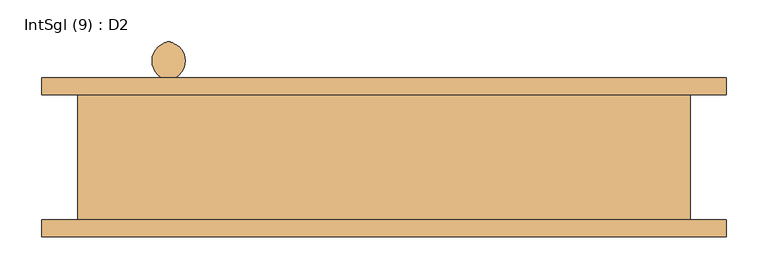
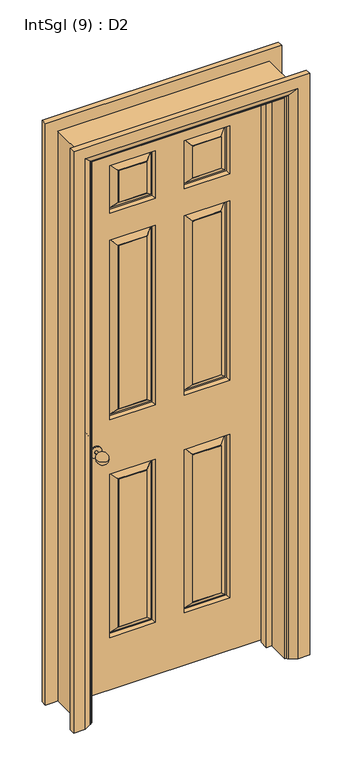
"""IFC4 building model written with IfcOpenShell, lengths in millimetres: door geometry, IntSgl (9) : D2."""

from ifc_helpers import new_model, si_unit, point, frame, origin, place, context, project, spatial, polyline, circle_curve, ellipse_curve, trimmed, outline, extrude, faceted_brep, source, transform, mapped, element, save
from ifc_brep_helpers import plane_surface, cylinder_surface, revolved_surface, advanced_brep


def intsgl_9_d2_8283ee4d(model_context):
    return source(origin(), model_context, "Body", "SolidModel", [
        advanced_brep(
        [(-253.0, 18.0, 900.0), (-258.0, -26.437411, 900.0), (-263.0, 18.0, 900.0), (-263.0, 33.0, 900.0), (-253.0, 33.0, 900.0), (-278.0, 37.0, 900.0), (-238.0, 37.0, 900.0), (-278.0, 33.0, 900.0), (-238.0, 33.0, 900.0)],
        [
            (0, 1, circle_curve(frame((-261.1884862, -3.5786495, 900.0), z_axis=(0.0, 0.0, -1.0), x_axis=(0.0, 1.0, 0.0)), 23.0800654)),
            (1, 2, circle_curve(frame((-254.8115138, -3.5786495, 900.0), z_axis=(0.0, 0.0, -1.0), x_axis=(0.0, 1.0, 0.0)), 23.0800654)),
            (2, 0, circle_curve(frame((-258.0, 18.0, 900.0), z_axis=(0.0, -1.0, 0.0), x_axis=(-1.0, 0.0, 0.0)), 5.0)),
            (0, 2, circle_curve(frame((-258.0, 18.0, 900.0), z_axis=(0.0, -1.0, 0.0), x_axis=(-1.0, 0.0, 0.0)), 5.0)),
            (2, 3),
            (3, 4, circle_curve(frame((-258.0, 33.0, 900.0), z_axis=(0.0, -1.0, 0.0), x_axis=(-1.0, 0.0, 0.0)), 5.0)),
            (4, 0),
            (4, 3, circle_curve(frame((-258.0, 33.0, 900.0), z_axis=(0.0, -1.0, 0.0), x_axis=(-1.0, 0.0, 0.0)), 5.0)),
            (5, 6, circle_curve(frame((-258.0, 37.0, 900.0), z_axis=(0.0, 1.0, 0.0), x_axis=(1.0, 0.0, 0.0)), 20.0)),
            (6, 5, circle_curve(frame((-258.0, 37.0, 900.0), z_axis=(0.0, 1.0, 0.0), x_axis=(1.0, 0.0, 0.0)), 20.0)),
            (7, 8, circle_curve(frame((-258.0, 33.0, 900.0), z_axis=(0.0, -1.0, 0.0), x_axis=(1.0, 0.0, 0.0)), 20.0)),
            (8, 7, circle_curve(frame((-258.0, 33.0, 900.0), z_axis=(0.0, -1.0, 0.0), x_axis=(1.0, 0.0, 0.0)), 20.0)),
            (6, 8),
            (7, 5),
        ],
        [
            revolved_surface(trimmed(ellipse_curve(frame((-254.8115138, -3.5786495, 900.0), z_axis=(0.0, 0.0, -1.0), x_axis=(0.0, 1.0, 0.0)), 23.0800654, 23.0800654), [point((-258.0, -26.437411, 900.0))], [point((-263.0, 18.0, 900.0))], True, "CARTESIAN"), (-258.0, 33.0, 900.0), (0.0, 1.0, 0.0)),
            cylinder_surface(frame((-258.0, 33.0, 900.0), z_axis=(0.0, 1.0, 0.0), x_axis=(-1.0, 0.0, 0.0)), 5.0),
            plane_surface(frame((-238.0, 37.0, 900.0), z_axis=(0.0, 1.0, 0.0), x_axis=(0.0, 0.0, 1.0))),
            plane_surface(frame((-238.0, 33.0, 900.0), z_axis=(0.0, -1.0, 0.0), x_axis=(0.0, 0.0, -1.0))),
            cylinder_surface(frame((-258.0, 33.0, 900.0), z_axis=(0.0, 1.0, 0.0), x_axis=(1.0, 0.0, 0.0)), 20.0),
        ],
        [
            (0, [[1, 2, 3]]),
            (0, [[-1, 4, -2]]),
            (1, [[5, 6, 7, -3]]),
            (1, [[-7, 8, -5, -4]]),
            (2, [[9, 10]]),
            (3, [[11, 12], [-8, -6]]),
            (4, [[13, -11, 14, -10]]),
            (4, [[-14, -12, -13, -9]]),
        ],
    ),
        advanced_brep(
        [(-253.0, 94.0, 900.0), (-263.0, 94.0, 900.0), (-258.0, 138.437411, 900.0), (-253.0, 79.0, 900.0), (-263.0, 79.0, 900.0), (-278.0, 75.0, 900.0), (-238.0, 75.0, 900.0), (-278.0, 79.0, 900.0), (-238.0, 79.0, 900.0)],
        [
            (0, 1, circle_curve(frame((-258.0, 94.0, 900.0), z_axis=(0.0, 1.0, 0.0), x_axis=(-1.0, 0.0, 0.0)), 5.0)),
            (1, 2, circle_curve(frame((-254.8115138, 115.5786495, 900.0), z_axis=(0.0, 0.0, -1.0), x_axis=(0.0, -1.0, 0.0)), 23.0800654)),
            (2, 0, circle_curve(frame((-261.1884862, 115.5786495, 900.0), z_axis=(0.0, 0.0, -1.0), x_axis=(0.0, -1.0, 0.0)), 23.0800654)),
            (1, 0, circle_curve(frame((-258.0, 94.0, 900.0), z_axis=(0.0, 1.0, 0.0), x_axis=(-1.0, 0.0, 0.0)), 5.0)),
            (0, 3),
            (3, 4, circle_curve(frame((-258.0, 79.0, 900.0), z_axis=(0.0, 1.0, 0.0), x_axis=(-1.0, 0.0, 0.0)), 5.0)),
            (4, 1),
            (4, 3, circle_curve(frame((-258.0, 79.0, 900.0), z_axis=(0.0, 1.0, 0.0), x_axis=(-1.0, 0.0, 0.0)), 5.0)),
            (5, 6, circle_curve(frame((-258.0, 75.0, 900.0), z_axis=(0.0, -1.0, 0.0), x_axis=(1.0, 0.0, 0.0)), 20.0)),
            (6, 5, circle_curve(frame((-258.0, 75.0, 900.0), z_axis=(0.0, -1.0, 0.0), x_axis=(1.0, 0.0, 0.0)), 20.0)),
            (7, 8, circle_curve(frame((-258.0, 79.0, 900.0), z_axis=(0.0, 1.0, 0.0), x_axis=(1.0, 0.0, 0.0)), 20.0)),
            (8, 7, circle_curve(frame((-258.0, 79.0, 900.0), z_axis=(0.0, 1.0, 0.0), x_axis=(1.0, 0.0, 0.0)), 20.0)),
            (5, 7),
            (8, 6),
        ],
        [
            revolved_surface(trimmed(ellipse_curve(frame((-254.8115138, 115.5786495, 900.0), z_axis=(0.0, 0.0, 1.0), x_axis=(0.0, -1.0, 0.0)), 23.0800654, 23.0800654), [point((-258.0, 138.437411, 900.0))], [point((-263.0, 94.0, 900.0))], True, "CARTESIAN"), (-258.0, 79.0, 900.0), (0.0, -1.0, 0.0)),
            cylinder_surface(frame((-258.0, 79.0, 900.0), z_axis=(0.0, -1.0, 0.0), x_axis=(-1.0, 0.0, 0.0)), 5.0),
            plane_surface(frame((-238.0, 75.0, 900.0), z_axis=(0.0, -1.0, 0.0), x_axis=(0.0, 0.0, 1.0))),
            plane_surface(frame((-238.0, 79.0, 900.0), z_axis=(0.0, 1.0, 0.0), x_axis=(0.0, 0.0, -1.0))),
            cylinder_surface(frame((-258.0, 79.0, 900.0), z_axis=(0.0, -1.0, 0.0), x_axis=(1.0, 0.0, 0.0)), 20.0),
        ],
        [
            (0, [[1, 2, 3]]),
            (0, [[-2, 4, -3]]),
            (1, [[-1, 5, 6, 7]]),
            (1, [[-4, -7, 8, -5]]),
            (2, [[9, 10]]),
            (3, [[11, 12], [-6, -8]]),
            (4, [[-9, 13, -12, 14]]),
            (4, [[-10, -14, -11, -13]]),
        ],
    ),
        faceted_brep([(-333.0, 37.0, 2058.0), (-333.0, 37.0, 8.0), (333.0, 37.0, 8.0), (333.0, 37.0, 2058.0), (-50.0, 37.0, 800.0), (-50.0, 37.0, 200.0), (-208.0, 37.0, 200.0), (-208.0, 37.0, 800.0), (208.0, 37.0, 800.0), (208.0, 37.0, 200.0), (50.0, 37.0, 200.0), (50.0, 37.0, 800.0), (-50.0, 37.0, 1658.0), (-50.0, 37.0, 1000.0), (-208.0, 37.0, 1000.0), (-208.0, 37.0, 1658.0), (208.0, 37.0, 1658.0), (208.0, 37.0, 1000.0), (50.0, 37.0, 1000.0), (50.0, 37.0, 1658.0), (-50.0, 37.0, 1933.0), (-50.0, 37.0, 1758.0), (-208.0, 37.0, 1758.0), (-208.0, 37.0, 1933.0), (208.0, 37.0, 1933.0), (208.0, 37.0, 1758.0), (50.0, 37.0, 1758.0), (50.0, 37.0, 1933.0), (-80.0, 37.0, 230.0), (-80.0, 37.0, 770.0), (-178.0, 37.0, 770.0), (-178.0, 37.0, 230.0), (178.0, 37.0, 230.0), (178.0, 37.0, 770.0), (80.0, 37.0, 770.0), (80.0, 37.0, 230.0), (-80.0, 37.0, 1030.0), (-80.0, 37.0, 1628.0), (-178.0, 37.0, 1628.0), (-178.0, 37.0, 1030.0), (178.0, 37.0, 1030.0), (178.0, 37.0, 1628.0), (80.0, 37.0, 1628.0), (80.0, 37.0, 1030.0), (-80.0, 37.0, 1788.0), (-80.0, 37.0, 1903.0), (-178.0, 37.0, 1903.0), (-178.0, 37.0, 1788.0), (178.0, 37.0, 1788.0), (178.0, 37.0, 1903.0), (80.0, 37.0, 1903.0), (80.0, 37.0, 1788.0), (-333.0, 75.0, 2058.0), (333.0, 75.0, 2058.0), (333.0, 75.0, 8.0), (-333.0, 75.0, 8.0), (50.0, 75.0, 800.0), (50.0, 75.0, 200.0), (208.0, 75.0, 200.0), (208.0, 75.0, 800.0), (-208.0, 75.0, 800.0), (-208.0, 75.0, 200.0), (-50.0, 75.0, 200.0), (-50.0, 75.0, 800.0), (50.0, 75.0, 1658.0), (50.0, 75.0, 1000.0), (208.0, 75.0, 1000.0), (208.0, 75.0, 1658.0), (-208.0, 75.0, 1658.0), (-208.0, 75.0, 1000.0), (-50.0, 75.0, 1000.0), (-50.0, 75.0, 1658.0), (50.0, 75.0, 1933.0), (50.0, 75.0, 1758.0), (208.0, 75.0, 1758.0), (208.0, 75.0, 1933.0), (-208.0, 75.0, 1933.0), (-208.0, 75.0, 1758.0), (-50.0, 75.0, 1758.0), (-50.0, 75.0, 1933.0), (80.0, 75.0, 230.0), (80.0, 75.0, 770.0), (178.0, 75.0, 770.0), (178.0, 75.0, 230.0), (-178.0, 75.0, 230.0), (-178.0, 75.0, 770.0), (-80.0, 75.0, 770.0), (-80.0, 75.0, 230.0), (80.0, 75.0, 1030.0), (80.0, 75.0, 1628.0), (178.0, 75.0, 1628.0), (178.0, 75.0, 1030.0), (-178.0, 75.0, 1030.0), (-178.0, 75.0, 1628.0), (-80.0, 75.0, 1628.0), (-80.0, 75.0, 1030.0), (80.0, 75.0, 1788.0), (80.0, 75.0, 1903.0), (178.0, 75.0, 1903.0), (178.0, 75.0, 1788.0), (-178.0, 75.0, 1788.0), (-178.0, 75.0, 1903.0), (-80.0, 75.0, 1903.0), (-80.0, 75.0, 1788.0), (80.0, 74.0, 230.0), (80.0, 74.0, 770.0), (58.0, 60.0, 208.0), (58.0, 60.0, 792.0), (78.0, 74.0, 772.0), (78.0, 74.0, 228.0), (53.0, 60.0, 797.0), (53.0, 60.0, 203.0), (178.0, 74.0, 770.0), (200.0, 60.0, 792.0), (180.0, 74.0, 772.0), (205.0, 60.0, 797.0), (178.0, 74.0, 230.0), (200.0, 60.0, 208.0), (180.0, 74.0, 228.0), (205.0, 60.0, 203.0), (-178.0, 74.0, 230.0), (-178.0, 74.0, 770.0), (-200.0, 60.0, 208.0), (-200.0, 60.0, 792.0), (-180.0, 74.0, 772.0), (-180.0, 74.0, 228.0), (-205.0, 60.0, 797.0), (-205.0, 60.0, 203.0), (-80.0, 74.0, 770.0), (-58.0, 60.0, 792.0), (-78.0, 74.0, 772.0), (-53.0, 60.0, 797.0), (-80.0, 74.0, 230.0), (-58.0, 60.0, 208.0), (-78.0, 74.0, 228.0), (-53.0, 60.0, 203.0), (80.0, 74.0, 1030.0), (80.0, 74.0, 1628.0), (58.0, 60.0, 1008.0), (58.0, 60.0, 1650.0), (78.0, 74.0, 1630.0), (78.0, 74.0, 1028.0), (53.0, 60.0, 1655.0), (53.0, 60.0, 1003.0), (178.0, 74.0, 1628.0), (200.0, 60.0, 1650.0), (180.0, 74.0, 1630.0), (205.0, 60.0, 1655.0), (178.0, 74.0, 1030.0), (200.0, 60.0, 1008.0), (180.0, 74.0, 1028.0), (205.0, 60.0, 1003.0), (-178.0, 74.0, 1030.0), (-178.0, 74.0, 1628.0), (-200.0, 60.0, 1008.0), (-200.0, 60.0, 1650.0), (-180.0, 74.0, 1630.0), (-180.0, 74.0, 1028.0), (-205.0, 60.0, 1655.0), (-205.0, 60.0, 1003.0), (-80.0, 74.0, 1628.0), (-58.0, 60.0, 1650.0), (-78.0, 74.0, 1630.0), (-53.0, 60.0, 1655.0), (-80.0, 74.0, 1030.0), (-58.0, 60.0, 1008.0), (-78.0, 74.0, 1028.0), (-53.0, 60.0, 1003.0), (80.0, 74.0, 1788.0), (80.0, 74.0, 1903.0), (58.0, 60.0, 1766.0), (58.0, 60.0, 1925.0), (78.0, 74.0, 1905.0), (78.0, 74.0, 1786.0), (53.0, 60.0, 1930.0), (53.0, 60.0, 1761.0), (178.0, 74.0, 1903.0), (200.0, 60.0, 1925.0), (180.0, 74.0, 1905.0), (205.0, 60.0, 1930.0), (178.0, 74.0, 1788.0), (200.0, 60.0, 1766.0), (180.0, 74.0, 1786.0), (205.0, 60.0, 1761.0), (-178.0, 74.0, 1788.0), (-178.0, 74.0, 1903.0), (-200.0, 60.0, 1766.0), (-200.0, 60.0, 1925.0), (-180.0, 74.0, 1905.0), (-180.0, 74.0, 1786.0), (-205.0, 60.0, 1930.0), (-205.0, 60.0, 1761.0), (-80.0, 74.0, 1903.0), (-58.0, 60.0, 1925.0), (-78.0, 74.0, 1905.0), (-53.0, 60.0, 1930.0), (-80.0, 74.0, 1788.0), (-58.0, 60.0, 1766.0), (-78.0, 74.0, 1786.0), (-53.0, 60.0, 1761.0), (-80.0, 38.0, 230.0), (-80.0, 38.0, 770.0), (-58.0, 52.0, 208.0), (-58.0, 52.0, 792.0), (-78.0, 38.0, 772.0), (-78.0, 38.0, 228.0), (-53.0, 52.0, 797.0), (-53.0, 52.0, 203.0), (-178.0, 38.0, 770.0), (-200.0, 52.0, 792.0), (-180.0, 38.0, 772.0), (-205.0, 52.0, 797.0), (-178.0, 38.0, 230.0), (-200.0, 52.0, 208.0), (-180.0, 38.0, 228.0), (-205.0, 52.0, 203.0), (178.0, 38.0, 230.0), (178.0, 38.0, 770.0), (200.0, 52.0, 208.0), (200.0, 52.0, 792.0), (180.0, 38.0, 772.0), (180.0, 38.0, 228.0), (205.0, 52.0, 797.0), (205.0, 52.0, 203.0), (80.0, 38.0, 770.0), (58.0, 52.0, 792.0), (78.0, 38.0, 772.0), (53.0, 52.0, 797.0), (80.0, 38.0, 230.0), (58.0, 52.0, 208.0), (78.0, 38.0, 228.0), (53.0, 52.0, 203.0), (-80.0, 38.0, 1030.0), (-80.0, 38.0, 1628.0), (-58.0, 52.0, 1008.0), (-58.0, 52.0, 1650.0), (-78.0, 38.0, 1630.0), (-78.0, 38.0, 1028.0), (-53.0, 52.0, 1655.0), (-53.0, 52.0, 1003.0), (-178.0, 38.0, 1628.0), (-200.0, 52.0, 1650.0), (-180.0, 38.0, 1630.0), (-205.0, 52.0, 1655.0), (-178.0, 38.0, 1030.0), (-200.0, 52.0, 1008.0), (-180.0, 38.0, 1028.0), (-205.0, 52.0, 1003.0), (178.0, 38.0, 1030.0), (178.0, 38.0, 1628.0), (200.0, 52.0, 1008.0), (200.0, 52.0, 1650.0), (180.0, 38.0, 1630.0), (180.0, 38.0, 1028.0), (205.0, 52.0, 1655.0), (205.0, 52.0, 1003.0), (80.0, 38.0, 1628.0), (58.0, 52.0, 1650.0), (78.0, 38.0, 1630.0), (53.0, 52.0, 1655.0), (80.0, 38.0, 1030.0), (58.0, 52.0, 1008.0), (78.0, 38.0, 1028.0), (53.0, 52.0, 1003.0), (-80.0, 38.0, 1788.0), (-80.0, 38.0, 1903.0), (-58.0, 52.0, 1766.0), (-58.0, 52.0, 1925.0), (-78.0, 38.0, 1905.0), (-78.0, 38.0, 1786.0), (-53.0, 52.0, 1930.0), (-53.0, 52.0, 1761.0), (-178.0, 38.0, 1903.0), (-200.0, 52.0, 1925.0), (-180.0, 38.0, 1905.0), (-205.0, 52.0, 1930.0), (-178.0, 38.0, 1788.0), (-200.0, 52.0, 1766.0), (-180.0, 38.0, 1786.0), (-205.0, 52.0, 1761.0), (178.0, 38.0, 1788.0), (178.0, 38.0, 1903.0), (200.0, 52.0, 1766.0), (200.0, 52.0, 1925.0), (180.0, 38.0, 1905.0), (180.0, 38.0, 1786.0), (205.0, 52.0, 1930.0), (205.0, 52.0, 1761.0), (80.0, 38.0, 1903.0), (58.0, 52.0, 1925.0), (78.0, 38.0, 1905.0), (53.0, 52.0, 1930.0), (80.0, 38.0, 1788.0), (58.0, 52.0, 1766.0), (78.0, 38.0, 1786.0), (53.0, 52.0, 1761.0)], [[[0, 1, 2, 3], [4, 5, 6, 7], [8, 9, 10, 11], [12, 13, 14, 15], [16, 17, 18, 19], [20, 21, 22, 23], [24, 25, 26, 27]], [[28, 29, 30, 31]], [[32, 33, 34, 35]], [[36, 37, 38, 39]], [[40, 41, 42, 43]], [[44, 45, 46, 47]], [[48, 49, 50, 51]], [[52, 53, 54, 55], [56, 57, 58, 59], [60, 61, 62, 63], [64, 65, 66, 67], [68, 69, 70, 71], [72, 73, 74, 75], [76, 77, 78, 79]], [[80, 81, 82, 83]], [[84, 85, 86, 87]], [[88, 89, 90, 91]], [[92, 93, 94, 95]], [[96, 97, 98, 99]], [[100, 101, 102, 103]], [[1, 0, 52, 55]], [[2, 1, 55, 54]], [[3, 2, 54, 53]], [[0, 3, 53, 52]], [[104, 105, 81, 80]], [[106, 107, 108, 109]], [[56, 110, 111, 57]], [[81, 105, 112, 82]], [[108, 107, 113, 114]], [[110, 56, 59, 115]], [[82, 112, 116, 83]], [[114, 113, 117, 118]], [[115, 59, 58, 119]], [[104, 80, 83, 116]], [[109, 108, 114, 118], [105, 104, 116, 112]], [[106, 109, 118, 117]], [[111, 110, 115, 119], [107, 106, 117, 113]], [[57, 111, 119, 58]], [[120, 121, 85, 84]], [[122, 123, 124, 125]], [[60, 126, 127, 61]], [[85, 121, 128, 86]], [[124, 123, 129, 130]], [[126, 60, 63, 131]], [[86, 128, 132, 87]], [[130, 129, 133, 134]], [[131, 63, 62, 135]], [[120, 84, 87, 132]], [[125, 124, 130, 134], [121, 120, 132, 128]], [[122, 125, 134, 133]], [[127, 126, 131, 135], [123, 122, 133, 129]], [[61, 127, 135, 62]], [[136, 137, 89, 88]], [[138, 139, 140, 141]], [[64, 142, 143, 65]], [[89, 137, 144, 90]], [[140, 139, 145, 146]], [[142, 64, 67, 147]], [[90, 144, 148, 91]], [[146, 145, 149, 150]], [[147, 67, 66, 151]], [[136, 88, 91, 148]], [[141, 140, 146, 150], [137, 136, 148, 144]], [[138, 141, 150, 149]], [[143, 142, 147, 151], [139, 138, 149, 145]], [[65, 143, 151, 66]], [[152, 153, 93, 92]], [[154, 155, 156, 157]], [[68, 158, 159, 69]], [[93, 153, 160, 94]], [[156, 155, 161, 162]], [[158, 68, 71, 163]], [[94, 160, 164, 95]], [[162, 161, 165, 166]], [[163, 71, 70, 167]], [[152, 92, 95, 164]], [[157, 156, 162, 166], [153, 152, 164, 160]], [[154, 157, 166, 165]], [[159, 158, 163, 167], [155, 154, 165, 161]], [[69, 159, 167, 70]], [[168, 169, 97, 96]], [[170, 171, 172, 173]], [[72, 174, 175, 73]], [[97, 169, 176, 98]], [[172, 171, 177, 178]], [[174, 72, 75, 179]], [[98, 176, 180, 99]], [[178, 177, 181, 182]], [[179, 75, 74, 183]], [[168, 96, 99, 180]], [[173, 172, 178, 182], [169, 168, 180, 176]], [[170, 173, 182, 181]], [[175, 174, 179, 183], [171, 170, 181, 177]], [[73, 175, 183, 74]], [[184, 185, 101, 100]], [[186, 187, 188, 189]], [[76, 190, 191, 77]], [[101, 185, 192, 102]], [[188, 187, 193, 194]], [[190, 76, 79, 195]], [[102, 192, 196, 103]], [[194, 193, 197, 198]], [[195, 79, 78, 199]], [[184, 100, 103, 196]], [[189, 188, 194, 198], [185, 184, 196, 192]], [[186, 189, 198, 197]], [[191, 190, 195, 199], [187, 186, 197, 193]], [[77, 191, 199, 78]], [[200, 201, 29, 28]], [[202, 203, 204, 205]], [[4, 206, 207, 5]], [[29, 201, 208, 30]], [[204, 203, 209, 210]], [[206, 4, 7, 211]], [[30, 208, 212, 31]], [[210, 209, 213, 214]], [[211, 7, 6, 215]], [[200, 28, 31, 212]], [[205, 204, 210, 214], [201, 200, 212, 208]], [[202, 205, 214, 213]], [[207, 206, 211, 215], [203, 202, 213, 209]], [[5, 207, 215, 6]], [[216, 217, 33, 32]], [[218, 219, 220, 221]], [[8, 222, 223, 9]], [[33, 217, 224, 34]], [[220, 219, 225, 226]], [[222, 8, 11, 227]], [[34, 224, 228, 35]], [[226, 225, 229, 230]], [[227, 11, 10, 231]], [[216, 32, 35, 228]], [[221, 220, 226, 230], [217, 216, 228, 224]], [[218, 221, 230, 229]], [[223, 222, 227, 231], [219, 218, 229, 225]], [[9, 223, 231, 10]], [[232, 233, 37, 36]], [[234, 235, 236, 237]], [[12, 238, 239, 13]], [[37, 233, 240, 38]], [[236, 235, 241, 242]], [[238, 12, 15, 243]], [[38, 240, 244, 39]], [[242, 241, 245, 246]], [[243, 15, 14, 247]], [[232, 36, 39, 244]], [[237, 236, 242, 246], [233, 232, 244, 240]], [[234, 237, 246, 245]], [[239, 238, 243, 247], [235, 234, 245, 241]], [[13, 239, 247, 14]], [[248, 249, 41, 40]], [[250, 251, 252, 253]], [[16, 254, 255, 17]], [[41, 249, 256, 42]], [[252, 251, 257, 258]], [[254, 16, 19, 259]], [[42, 256, 260, 43]], [[258, 257, 261, 262]], [[259, 19, 18, 263]], [[248, 40, 43, 260]], [[253, 252, 258, 262], [249, 248, 260, 256]], [[250, 253, 262, 261]], [[255, 254, 259, 263], [251, 250, 261, 257]], [[17, 255, 263, 18]], [[264, 265, 45, 44]], [[266, 267, 268, 269]], [[20, 270, 271, 21]], [[45, 265, 272, 46]], [[268, 267, 273, 274]], [[270, 20, 23, 275]], [[46, 272, 276, 47]], [[274, 273, 277, 278]], [[275, 23, 22, 279]], [[264, 44, 47, 276]], [[269, 268, 274, 278], [265, 264, 276, 272]], [[266, 269, 278, 277]], [[271, 270, 275, 279], [267, 266, 277, 273]], [[21, 271, 279, 22]], [[280, 281, 49, 48]], [[282, 283, 284, 285]], [[24, 286, 287, 25]], [[49, 281, 288, 50]], [[284, 283, 289, 290]], [[286, 24, 27, 291]], [[50, 288, 292, 51]], [[290, 289, 293, 294]], [[291, 27, 26, 295]], [[280, 48, 51, 292]], [[285, 284, 290, 294], [281, 280, 292, 288]], [[282, 285, 294, 293]], [[287, 286, 291, 295], [283, 282, 293, 289]], [[25, 287, 295, 26]]]),
        faceted_brep([(-335.0, 75.0, 0.0), (-335.0, -75.0, 0.0), (-367.0, -75.0, 0.0), (-367.0, 75.0, 0.0), (-335.0, 75.0, 2060.0), (-335.0, -75.0, 2060.0), (-367.0, -75.0, 2092.0), (-367.0, 75.0, 2092.0), (335.0, 75.0, 0.0), (367.0, 75.0, 0.0), (367.0, -75.0, 0.0), (335.0, -75.0, 0.0), (335.0, 75.0, 2060.0), (367.0, 75.0, 2092.0), (367.0, -75.0, 2092.0), (335.0, -75.0, 2060.0)], [[[0, 1, 2, 3]], [[1, 0, 4, 5]], [[2, 1, 5, 6]], [[3, 2, 6, 7]], [[0, 3, 7, 4]], [[8, 9, 10, 11]], [[12, 13, 9, 8]], [[13, 14, 10, 9]], [[14, 15, 11, 10]], [[15, 12, 8, 11]], [[5, 4, 12, 15]], [[6, 5, 15, 14]], [[7, 6, 14, 13]], [[4, 7, 13, 12]]]),
        extrude(outline(polyline([(0.0, -335.0), (0.0, -316.0), (2041.0, -316.0), (2041.0, 316.0), (0.0, 316.0), (0.0, 335.0), (2060.0, 335.0), (2060.0, -335.0), (0.0, -335.0)])), frame((0.0, 3.0, 0.0), z_axis=(0.0, 1.0, 0.0), x_axis=(0.0, 0.0, 1.0)), (0.0, 0.0, 1.0), 32.0),
        advanced_brep(
        [(-410.0, -95.0, 0.0), (-410.0, -75.0, 0.0), (-340.0, -75.0, 0.0), (-344.0, -81.0, 0.0), (-370.0, -95.0, 0.0), (-410.0, -95.0, 2135.0), (-410.0, -75.0, 2135.0), (410.0, -75.0, 2135.0), (410.0, -75.0, 0.0), (340.0, -75.0, 0.0), (340.0, -75.0, 2065.0), (-340.0, -75.0, 2065.0), (-344.0, -81.0, 2069.0), (-370.0, -95.0, 2095.0), (370.0, -95.0, 2095.0), (370.0, -95.0, 0.0), (410.0, -95.0, 0.0), (410.0, -95.0, 2135.0), (344.0, -81.0, 0.0), (344.0, -81.0, 2069.0)],
        [
            (0, 1),
            (1, 2),
            (2, 3, circle_curve(frame((-348.0, -74.0, 0.0), z_axis=(0.0, 0.0, -1.0), x_axis=(-1.0, 0.0, 0.0)), 8.0622577)),
            (3, 4),
            (4, 0),
            (0, 5),
            (5, 6),
            (6, 1),
            (6, 7),
            (7, 8),
            (8, 9),
            (9, 10),
            (10, 11),
            (11, 2),
            (11, 12, ellipse_curve(frame((-348.0, -74.0, 2073.0), z_axis=(-0.7071067811865475, 0.0, -0.7071067811865475), x_axis=(0.7071067811865474, 0.0, -0.7071067811865476)), 11.4017543, 8.0622577)),
            (12, 3),
            (12, 13),
            (13, 4),
            (13, 14),
            (14, 15),
            (15, 16),
            (16, 17),
            (17, 5),
            (7, 17),
            (16, 8),
            (15, 18),
            (18, 9, circle_curve(frame((348.0, -74.0, 0.0), z_axis=(0.0, 0.0, -1.0), x_axis=(1.0, 0.0, 0.0)), 8.0622577)),
            (19, 10, ellipse_curve(frame((348.0, -74.0, 2073.0), z_axis=(0.7071067811865475, 0.0, -0.7071067811865475), x_axis=(0.7071067811865474, 0.0, 0.7071067811865476)), 11.4017543, 8.0622577)),
            (18, 19),
            (14, 19),
            (19, 12),
        ],
        [
            plane_surface(frame((-340.0, -75.0, 0.0), z_axis=(0.0, 0.0, -1.0), x_axis=(0.0, -1.0, 0.0))),
            plane_surface(frame((-410.0, -95.0, 0.0), z_axis=(-1.0, 0.0, 0.0), x_axis=(0.0, 0.0, 1.0))),
            plane_surface(frame((-410.0, -75.0, 0.0), z_axis=(0.0, 1.0, 0.0), x_axis=(0.0, 0.0, 1.0))),
            cylinder_surface(frame((-348.0, -74.0, 0.0), z_axis=(0.0, 0.0, -1.0), x_axis=(-1.0, 0.0, 0.0)), 8.0622577),
            plane_surface(frame((-344.0, -81.0, 0.0), z_axis=(0.4740998230350183, -0.8804710999221749, 0.0), x_axis=(0.0, 0.0, 1.0))),
            plane_surface(frame((-370.0, -95.0, 0.0), z_axis=(0.0, -1.0, 0.0), x_axis=(0.0, 0.0, 1.0))),
            plane_surface(frame((410.0, -95.0, 2135.0), z_axis=(1.0, 0.0, 0.0), x_axis=(0.0, 0.0, -1.0))),
            plane_surface(frame((340.0, -75.0, 0.0), z_axis=(0.0, 0.0, -1.0), x_axis=(0.0, -1.0, 0.0))),
            cylinder_surface(frame((348.0, -74.0, 2065.0), z_axis=(0.0, 0.0, 1.0), x_axis=(1.0, 0.0, 0.0)), 8.0622577),
            plane_surface(frame((344.0, -81.0, 2069.0), z_axis=(-0.4740998230350183, -0.8804710999221749, 0.0), x_axis=(0.0, 0.0, -1.0))),
            plane_surface(frame((-410.0, -95.0, 2135.0), z_axis=(0.0, 0.0, 1.0), x_axis=(1.0, 0.0, 0.0))),
            cylinder_surface(frame((-340.0, -74.0, 2073.0), z_axis=(-1.0, 0.0, 0.0), x_axis=(0.0, 0.0, 1.0)), 8.0622577),
            plane_surface(frame((-344.0, -81.0, 2069.0), z_axis=(0.0, -0.8804710999221749, -0.4740998230350183), x_axis=(1.0, 0.0, 0.0))),
        ],
        [
            (0, [[1, 2, 3, 4, 5]]),
            (1, [[-1, 6, 7, 8]]),
            (2, [[-2, -8, 9, 10, 11, 12, 13, 14]]),
            (3, [[-3, -14, 15, 16]]),
            (4, [[-4, -16, 17, 18]]),
            (5, [[-5, -18, 19, 20, 21, 22, 23, -6]]),
            (6, [[24, -22, 25, -10]]),
            (7, [[-21, 26, 27, -11, -25]]),
            (8, [[28, -12, -27, 29]]),
            (9, [[30, -29, -26, -20]]),
            (10, [[-7, -23, -24, -9]]),
            (11, [[-15, -13, -28, 31]]),
            (12, [[-17, -31, -30, -19]]),
        ],
    ),
        advanced_brep(
        [(410.0, 95.0, 0.0), (410.0, 75.0, 0.0), (340.0, 75.0, 0.0), (344.0, 81.0, 0.0), (370.0, 95.0, 0.0), (410.0, 95.0, 2135.0), (410.0, 75.0, 2135.0), (-410.0, 75.0, 2135.0), (-410.0, 75.0, 0.0), (-340.0, 75.0, 0.0), (-340.0, 75.0, 2065.0), (340.0, 75.0, 2065.0), (344.0, 81.0, 2069.0), (370.0, 95.0, 2095.0), (-370.0, 95.0, 2095.0), (-370.0, 95.0, 0.0), (-410.0, 95.0, 0.0), (-410.0, 95.0, 2135.0), (-344.0, 81.0, 0.0), (-344.0, 81.0, 2069.0)],
        [
            (0, 1),
            (1, 2),
            (2, 3, circle_curve(frame((348.0, 74.0, 0.0), z_axis=(0.0, 0.0, -1.0), x_axis=(1.0, 0.0, 0.0)), 8.0622577)),
            (3, 4),
            (4, 0),
            (0, 5),
            (5, 6),
            (6, 1),
            (6, 7),
            (7, 8),
            (8, 9),
            (9, 10),
            (10, 11),
            (11, 2),
            (11, 12, ellipse_curve(frame((348.0, 74.0, 2073.0), z_axis=(0.7071067811865475, 0.0, -0.7071067811865475), x_axis=(-0.7071067811865474, 0.0, -0.7071067811865476)), 11.4017543, 8.0622577)),
            (12, 3),
            (12, 13),
            (13, 4),
            (13, 14),
            (14, 15),
            (15, 16),
            (16, 17),
            (17, 5),
            (7, 17),
            (16, 8),
            (15, 18),
            (18, 9, circle_curve(frame((-348.0, 74.0, 0.0), z_axis=(0.0, 0.0, -1.0), x_axis=(-1.0, 0.0, 0.0)), 8.0622577)),
            (19, 10, ellipse_curve(frame((-348.0, 74.0, 2073.0), z_axis=(-0.7071067811865475, 0.0, -0.7071067811865475), x_axis=(-0.7071067811865474, 0.0, 0.7071067811865476)), 11.4017543, 8.0622577)),
            (18, 19),
            (14, 19),
            (19, 12),
        ],
        [
            plane_surface(frame((340.0, 75.0, 0.0), z_axis=(0.0, 0.0, -1.0), x_axis=(0.0, 1.0, 0.0))),
            plane_surface(frame((410.0, 95.0, 0.0), z_axis=(1.0, 0.0, 0.0), x_axis=(0.0, 0.0, 1.0))),
            plane_surface(frame((410.0, 75.0, 0.0), z_axis=(0.0, -1.0, 0.0), x_axis=(0.0, 0.0, 1.0))),
            cylinder_surface(frame((348.0, 74.0, 0.0), z_axis=(0.0, 0.0, -1.0), x_axis=(1.0, 0.0, 0.0)), 8.0622577),
            plane_surface(frame((344.0, 81.0, 0.0), z_axis=(-0.4740998230350183, 0.8804710999221749, 0.0), x_axis=(0.0, 0.0, 1.0))),
            plane_surface(frame((370.0, 95.0, 0.0), z_axis=(0.0, 1.0, 0.0), x_axis=(0.0, 0.0, 1.0))),
            plane_surface(frame((-410.0, 95.0, 2135.0), z_axis=(-1.0, 0.0, 0.0), x_axis=(0.0, 0.0, -1.0))),
            plane_surface(frame((-340.0, 75.0, 0.0), z_axis=(0.0, 0.0, -1.0), x_axis=(0.0, 1.0, 0.0))),
            cylinder_surface(frame((-348.0, 74.0, 2065.0), z_axis=(0.0, 0.0, 1.0), x_axis=(-1.0, 0.0, 0.0)), 8.0622577),
            plane_surface(frame((-344.0, 81.0, 2069.0), z_axis=(0.4740998230350183, 0.8804710999221749, 0.0), x_axis=(0.0, 0.0, -1.0))),
            plane_surface(frame((410.0, 95.0, 2135.0), z_axis=(0.0, 0.0, 1.0), x_axis=(-1.0, 0.0, 0.0))),
            cylinder_surface(frame((340.0, 74.0, 2073.0), z_axis=(1.0, 0.0, 0.0), x_axis=(0.0, 0.0, 1.0)), 8.0622577),
            plane_surface(frame((344.0, 81.0, 2069.0), z_axis=(0.0, 0.8804710999221749, -0.4740998230350183), x_axis=(-1.0, 0.0, 0.0))),
        ],
        [
            (0, [[1, 2, 3, 4, 5]]),
            (1, [[-1, 6, 7, 8]]),
            (2, [[-2, -8, 9, 10, 11, 12, 13, 14]]),
            (3, [[-3, -14, 15, 16]]),
            (4, [[-4, -16, 17, 18]]),
            (5, [[-5, -18, 19, 20, 21, 22, 23, -6]]),
            (6, [[24, -22, 25, -10]]),
            (7, [[-21, 26, 27, -11, -25]]),
            (8, [[28, -12, -27, 29]]),
            (9, [[30, -29, -26, -20]]),
            (10, [[-7, -23, -24, -9]]),
            (11, [[-15, -13, -28, 31]]),
            (12, [[-17, -31, -30, -19]]),
        ],
    ),
    ])


if __name__ == "__main__":
    model = new_model("IFC4")
    model_context = context("Model", 3, world=origin())
    ifc_project = project(units=[si_unit("LENGTHUNIT", "METRE", prefix="MILLI")], contexts=[model_context])
    site = spatial("IfcSite", under=ifc_project)
    building = spatial("IfcBuilding", under=site)
    placement = place(None, origin())
    intsgl_9_d2_shape = intsgl_9_d2_8283ee4d(model_context)
    element("IfcDoor", 1, ObjectType="IntSgl (9) : D2", at=placement, inside=building, context=model_context, shape_type="MappedRepresentation", body=[
        mapped(intsgl_9_d2_shape, transform((0.0, 0.0, 0.0), x_axis=(1.0, 0.0, 0.0), y_axis=(0.0, 1.0, 0.0), z_axis=(0.0, 0.0, 1.0))),
    ])
    save(model, "model.ifc")

# Revit data of these elements
# Type "IntSgl (9) : D2"
#   Type Mark = "50"
#   Operation = "SingleSwingRight"
#   Manufacturer = "Revit"
#   Keynote = "L20"
#   UnderCut = 8 mm
#   Tolerance = 2 mm
#   Thickness = 38 mm
#   Structural Tolerance = 8 mm
#   StopDepth = 32 mm
#   Stop Thickness = 19 mm
#   Stile Top Rail = 125 mm
#   Stile Shutting = 125 mm
#   Stile Muntin Rail = 100 mm
#   Stile Lock Rail = 200 mm
#   Stile Intermediate/Frieze = 100 mm
#   Stile Hanging = 125 mm
#   Stile Bottom Rail = 200 mm
#   Rough Width = 750 mm
#   Rough Height = 2100 mm
#   Height to Top Lock Rail = 1000 mm
#   Handle Z Distance = 900 mm
#   Handle X Distance = 75 mm
#   Frame Thickness = 32 mm
#   Door Panel Width = 666 mm
#   Height = 2100 mm
#   Width = 750 mm
#   Door Panel Thickness = 38 mm
#   Door Panel Offset = 0 mm
#   Door Panel Height = 2050 mm
#   Architrave Setback = 5 mm
#   Vis - Ironmongery = yes
#   Material Ironmongery = Door - Handle
#   Material Frame = Door - Frame/Mullion
#   Material Door = Door - Panel
#   Material Architrave = Door - Architrave
#   Function = (empty or 0)
#   Wall Closure = (empty or 0)
# Element 1 (IfcDoor, "IntSgl (9) : D2")
#   Materials on its faces: "Door - Panel", "Door - Architrave", "Door - Frame/Mullion", "Door - Handle"
# Materials
#   "Door - Handle": colour RGB 247 247 247, transparency 0
#   "Door - Frame/Mullion": colour RGB 212 179 113, transparency 0
#   "Door - Panel": colour RGB 154 90 5, transparency 0
#   "Door - Architrave": colour RGB 154 90 5, transparency 0
